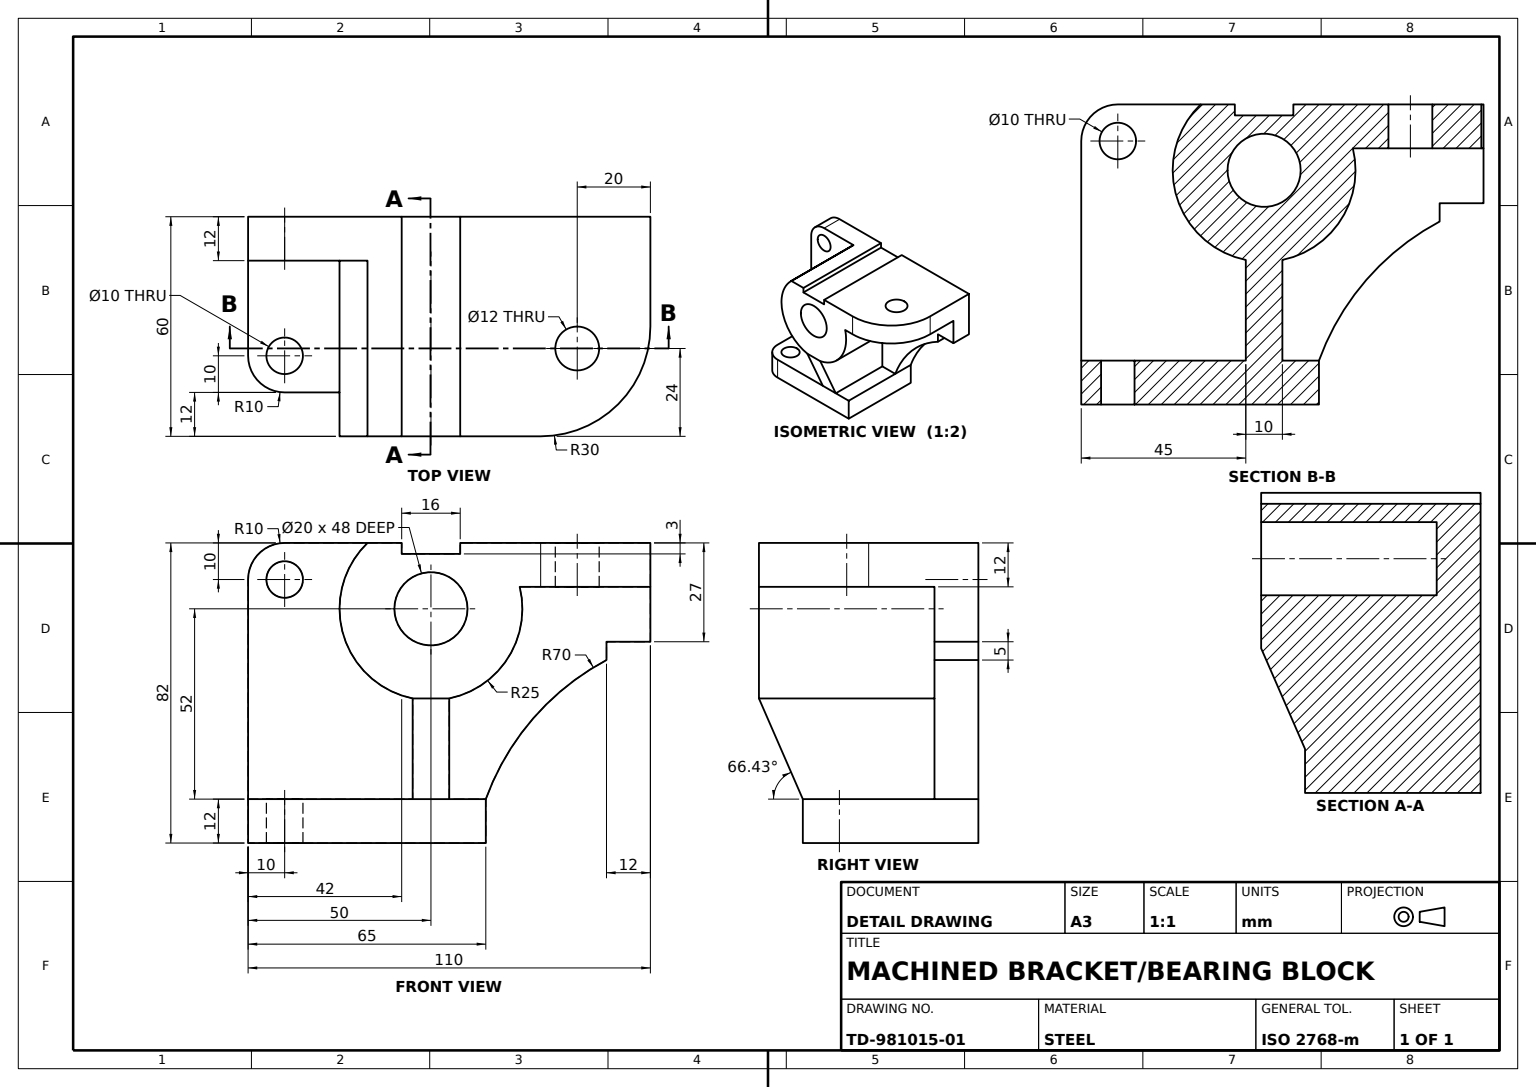
SolidWorks part; units mm, degrees
material "Plain Carbon Steel"
ref_plane "Front Plane" through (0, 0, 0) normal (0, 0, 1) x (1, 0, 0)
ref_plane "Top Plane" through (0, 0, 0) normal (0, 1, 0) x (1, 0, 0)
ref_plane "Right Plane" through (0, 0, 0) normal (1, 0, 0) x (0, 0, -1)
sketch "Base Plate Sketch" plane through (0, 0, 0) normal (0, 1, 0) x (1, 0, 0)
  line L1 (-32.5, -24) -> (32.5, -24)
  line L2 (-32.5, -24) -> (-32.5, 24)
  line L3 (-32.5, 24) -> (32.5, 24)
  line L4 (32.5, -24) -> (32.5, 24)
  line L5 (-32.5, -24) -> (32.5, 24) construction
  line L6 (-32.5, 24) -> (32.5, -24) construction
  point P0 (0, 0)
  dimension "D1" = 65
  dimension "D2" = 48
extrude "Base Plate" add sketch "Base Plate Sketch" along normal blind 12
sketch "Upper Block Sketch" plane through (0, 0, -24) normal (0, 0, -1) x (-1, 0, 0)
  line L0 (32.5, 12) -> (32.5, 82)
  line L1 (32.5, 82) -> (-77.5, 82)
  line L2 (-77.5, 82) -> (-77.5, 55)
  line L3 (-77.5, 55) -> (-65.5, 55)
  line L4 (-65.5, 55) -> (-65.5, 50)
  line L5 (-32.5, 12) -> (32.5, 12)
  arc A0 (-65.5, 50) -> (-32.5, 12) centre (-98.319, -11.8297) cw
  dimension "D1" = 70
  dimension "D5" = 70
  dimension "D2" = 110
  dimension "D3" = 27
  dimension "D4" = 12
  dimension "D6" = 5
extrude "Upper Block" add sketch "Upper Block Sketch" against normal blind 12
sketch "Support Web Sketch" plane through (0, 0, -12) normal (0, 0, 1) x (1, 0, 0)
  line L0 (-32.5, 82) -> (77.5, 82) construction
  line L1 (0.1506, 82) -> (34.8494, 82)
  arc A0 (0.1506, 82) -> (34.8494, 82) centre (17.5, 64) ccw
  circle A1 centre (17.5, 64) radius 10
  dimension "D1" = 50
  dimension "D2" = 20
  dimension "D3" = 18
  dimension "D4" = 15
extrude "Support Web" add sketch "Support Web Sketch" along normal blind 48
sketch "Top Slot Sketch" plane through (0, 82, 0) normal (0, 1, 0) x (1, 0, 0)
  line L1 (34.8494, -36) -> (0.1506, -36) construction
  line L2 (-32.5, 24) -> (77.5, 24) construction
  line L3 (9.5, 24) -> (25.5, 24)
  line L4 (9.5, 24) -> (9.5, -36)
  line L5 (9.5, -36) -> (25.5, -36)
  line L6 (25.5, 24) -> (25.5, -36)
  dimension "D1" = 16
  dimension "D2" = 42
extrude "Top Slot" cut sketch "Top Slot Sketch" against normal blind 3
sketch "Hub Boss Sketch" plane through (0, 82, 0) normal (0, 1, 0) x (1, 0, 0)
  line L0 (34.8494, -36) -> (25.5, -36) construction
  line L1 (25.5, 24) -> (77.5, 24)
  line L2 (25.5, 24) -> (25.5, -36)
  line L3 (25.5, -36) -> (77.5, -36)
  line L4 (77.5, 24) -> (77.5, -36)
  circle A0 centre (57.5, -12) radius 6
  dimension "D3" = 12
  dimension "D1" = 0
  dimension "D2" = 52
  dimension "D4" = 20
  dimension "D5" = 24
extrude "Hub Boss" add sketch "Hub Boss Sketch" against normal blind 12
fillet "Hub Round R30" radius 30 1 edges at (77.5, 76, 36)
sketch "Upper Mounting Hole Sketch" plane through (0, 0, -12) normal (0, 0, 1) x (1, 0, 0)
  line L0 (-32.5, 12) -> (-32.5, 82) construction
  line L1 (-32.5, 82) -> (0.1506, 82) construction
  circle A0 centre (-22.5, 72) radius 5
  dimension "D1" = 10
  dimension "D2" = 10
  dimension "D3" = 10
extrude "Upper Mounting Hole" cut sketch "Upper Mounting Hole Sketch" against normal blind 12
sketch "Base Mounting Hole Sketch" plane through (0, 12, 0) normal (0, 1, 0) x (1, 0, 0)
  line L0 (-32.5, -24) -> (32.5, -24) construction
  line L1 (-32.5, 12) -> (-32.5, -24) construction
  circle A0 centre (-22.5, -14) radius 5
  dimension "D1" = 10
  dimension "D2" = 10
  dimension "D3" = 10
extrude "Base Mounting Hole" cut sketch "Base Mounting Hole Sketch" against normal blind 12
fillet "Upper Block Fillet R10" radius 10 2 edges at (-32.5, 6, 24) (-32.5, 82, -18)
sketch "Side Support Sketch" plane through (0, 0, -12) normal (0, 0, 1) x (1, 0, 0)
  line L0 (17.5, 12) -> (12.5, 12)
  line L1 (-22.5, 12) -> (32.5, 12) construction
  line L3 (12.5, 12) -> (12.5, 39.5051)
  line L5 (22.5, 39.5051) -> (22.5, 12)
  line L6 (22.5, 12) -> (17.5, 12)
  arc A0 (12.5, 39.5051) -> (22.5, 39.5051) centre (17.5, 64) ccw
  arc A1 (0.1506, 82) -> (41.7693, 70) centre (17.5, 64) ccw construction
  dimension "D2" = 25
  dimension "D1" = 10
  dimension "D3" = 27.5051
  dimension "D4" = 5
extrude "Side Support" add sketch "Side Support Sketch" along normal blind 48
sketch "Side Relief Sketch" plane through (22.5, 0, 0) normal (1, 0, 0) x (0, 0, -1)
  line L0 (-36, 39.5051) -> (-24, 12)
  line L1 (-24, 12) -> (-36, 12)
  line L2 (-36, 12) -> (-36, 39.5051)
extrude "Side Relief Cut" cut sketch "Side Relief Sketch" against normal blind 48
